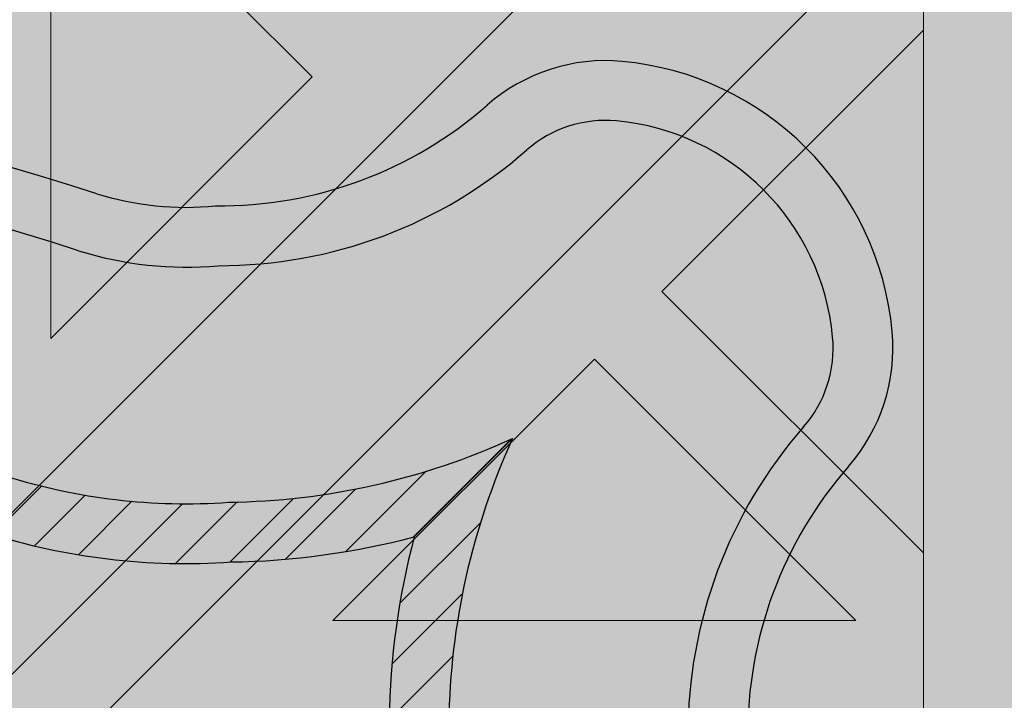
# Model space of a CAD drawing. Units: inches. Extents: x 844 to 2234, y 346 to 1084.
# Tile 20 of 93: x 1124.911 to 1127.536, y 703.246 to 705.06. Entities that reach past the tile are written whole.
import ezdxf

# ---------------------------------------------------------------- set-up
doc = ezdxf.new("R2010")
doc.units = ezdxf.units.IN
doc.header["$MEASUREMENT"] = 0
for name, color, linetype, lineweight in [('A-ANNO-DIMS', 2, 'Continuous', 18), ('furniture', 8, 'Continuous', 18), ('RA-AP-01$0$INT', 35, 'Continuous', 5)]:
    doc.layers.add(name, color=color, linetype=linetype, lineweight=lineweight)
doc.layers.add('RA-AP-01$0$FURN', color=3, linetype='Continuous')
doc.layers.add('RA-AP-01$0$WOOD', color=64, linetype='Continuous')
doc.styles.get("Standard").update_dxf_attribs({"font": 'arial.ttf'})
doc.dimstyles.get("Standard").update_dxf_attribs({"dimtxt": 6, "dimasz": 3, "dimexe": 0.18, "dimexo": 0.0625, "dimgap": 0.09, "dimtad": 0, "dimtih": 1, "dimtoh": 1, "dimdec": 1, "dimzin": 0, "dimdsep": 46, "dimlunit": 3, "dimtxsty": 'Standard', "dimblk": 'ARCHTICK', "dimcen": 0.09, "dimadec": 0, "dimazin": 0, "dimtfac": 1, "dimtdec": 1, "dimtofl": 0, "dimtmove": 0, "dimatfit": 3, "dimfxl": 1, "dimtolj": 1, "dimtzin": 0, "dimarcsym": 0})

# ---------------------------------------------------------------- blocks, each defined once
blk = doc.blocks.new('A$C18D01794')
at = {"layer": 'RA-AP-01$0$INT'}
blk.add_hatch(color=256, dxfattribs=at).paths.add_polyline_path([(4.505206456958071, -7.906712009588039), (5.305206456958072, -7.906712009588039), (5.305206456958072, -7.106712009588038), (5.255206456951893, -7.106712009588036), (5.25520645694868, -7.856712009570104), (4.555206456959269, -7.856712009588616), (4.555206456956052, -7.106712009588038), (4.505206456958073, -7.106712009588038)])
h = blk.add_hatch(color=256, dxfattribs=at)
h.paths.add_polyline_path([(4.585917135068448, -7.856712009587804), (4.614201406330596, -7.856712009587056), (4.668846067270487, -7.802067348644738), (4.723490728212344, -7.856712009584164), (4.771774999457151, -7.856712009582887), (4.826419660396886, -7.80206734864072), (4.862780050090322, -7.838427738332541), (4.844495778842715, -7.856712009580965), (4.862780050090411, -7.856712009580482), (4.905206456960182, -7.814285602707865), (4.947632863832445, -7.856712009578238), (4.965917135079675, -7.856712009577755), (4.947632863831759, -7.838427738330656), (4.983993253523576, -7.802067348637219), (5.038637914464627, -7.856712009575829), (5.08692218571208, -7.856712009574554), (5.141566846649976, -7.802067348634224), (5.196211507589851, -7.856712009571666), (5.224495778822615, -7.856712009570916), (4.905206456953975, -7.537422687702283)])
h.paths.add_polyline_path([(4.895206456956031, -7.575706958950402), (4.895206456958921, -7.684996280828174), (4.840561796018589, -7.630351619890275)], flags=16)
h.paths.add_polyline_path([(4.915206456955638, -7.575706958949956), (4.969851117895509, -7.630351619887399), (4.915206456957609, -7.684996280827732)], flags=16)
h.paths.add_polyline_path([(4.826419660395175, -7.644493755514321), (4.881064321335613, -7.699138416452331), (4.771774999456703, -7.69913841645522)], flags=16)
h.paths.add_polyline_path([(4.983993253519558, -7.644493755510815), (5.038637914460456, -7.699138416449285), (4.929348592581548, -7.69913841645126)], flags=16)
h.paths.add_polyline_path([(4.881064321336025, -7.719138416452334), (4.826419660397532, -7.773783077393256), (4.771774999457062, -7.719138416455217)], flags=16)
h.paths.add_polyline_path([(4.929348592582019, -7.71913841645126), (5.038637914460982, -7.719138416449284), (4.983993253522945, -7.773783077389749)], flags=16)
h.paths.add_polyline_path([(4.895206456960191, -7.733280552075633), (4.895206456962115, -7.806001331460164), (4.876922185715016, -7.824285602708492), (4.840561796021581, -7.787925213016675)], flags=16)
h.paths.add_polyline_path([(4.915206456958487, -7.733280552075187), (4.969851117899527, -7.787925213013798), (4.933490728206909, -7.824285602708034), (4.9152064569598, -7.806001331461736)], flags=16)
h.paths.add_polyline_path([(4.757632863832376, -7.733280552079264), (4.812277524772842, -7.787925213017304), (4.757632863834348, -7.842569873958233)], flags=16)
h.paths.add_polyline_path([(4.737632863832376, -7.73328055207979), (4.737632863834348, -7.842569873958701), (4.682988202893906, -7.787925213020692)], flags=16)
h.paths.add_polyline_path([(5.05278005008503, -7.733280552072701), (5.052780050087917, -7.842569873951664), (4.998135389146995, -7.787925213013169)], flags=16)
h.paths.add_polyline_path([(5.072780050085024, -7.733280552072333), (5.127424711025931, -7.787925213010806), (5.072780050087916, -7.842569873951244)], flags=16)
h.paths.add_polyline_path([(4.935917135072783, -7.506712009583784), (5.255206456948811, -7.826001331459767), (5.255206456948932, -7.797717060211899), (5.200561796010279, -7.743072399273238), (5.255206456949403, -7.688427738334128), (5.25520645694961, -7.640143467086677), (5.200561796009787, -7.585498806146837), (5.236922185702417, -7.549138416454212), (5.255206456949919, -7.56742268770172), (5.255206456949998, -7.549138416454178), (5.212780050078687, -7.506712009583814), (5.25520645695036, -7.464285602712145), (5.255206456950438, -7.446001331464763), (5.236922185702424, -7.464285602712779), (5.200561796009796, -7.427925213020149), (5.255206456950753, -7.373280552079203), (5.25520645695096, -7.324996280834394), (5.200561796010322, -7.270351619893748), (5.255206456951428, -7.215706958952649), (5.255206456951547, -7.187422687705071)])
h.paths.add_polyline_path([(5.042988202883395, -7.42792521302065), (5.097632863823085, -7.373280552080975), (5.097632863822622, -7.482569873959883)], flags=16)
h.paths.add_polyline_path([(5.028846067259663, -7.442067348644384), (5.083490728198774, -7.496712009583504), (4.974201406321001, -7.496712009583035)], flags=16)
h.paths.add_polyline_path([(5.117632863823087, -7.37328055208089), (5.172277524762331, -7.42792521302015), (5.11763286382262, -7.482569873959851)], flags=16)
h.paths.add_polyline_path([(5.08349072819877, -7.516712009582191), (5.028846067259652, -7.571356670521302), (4.974201406320998, -7.516712009582638)], flags=16)
h.paths.add_polyline_path([(5.131774999446817, -7.35913841645716), (5.186419660386065, -7.413783077396415), (5.241064321325782, -7.359138416456712)], flags=17)
h.paths.add_polyline_path([(5.131774999446228, -7.496712009583703), (5.186419660386065, -7.442067348643883), (5.222780050079488, -7.478427738337313), (5.204495778832781, -7.496712009584014)], flags=16)
h.paths.add_polyline_path([(5.097632863822613, -7.530854145205813), (5.097632863823061, -7.640143467084723), (5.042988202883383, -7.585498806145032)], flags=16)
h.paths.add_polyline_path([(5.131774999446899, -7.339138416457162), (5.241064321325809, -7.339138416456712), (5.186419660386591, -7.284493755517479)], flags=17)
h.paths.add_polyline_path([(5.131774999446226, -7.516712009581999), (5.204495778830767, -7.516712009581702), (5.22278005007868, -7.534996280829206), (5.186419660386049, -7.571356670521828)], flags=16)
h.paths.add_polyline_path([(5.11763286382262, -7.530854145205852), (5.17227752476232, -7.585498806145562), (5.117632863823064, -7.64014346708481)], flags=16)
h.paths.add_polyline_path([(5.186419660386069, -7.599640941770585), (5.241064321325754, -7.654285602710281), (5.131774999446791, -7.654285602709814)], flags=16)
h.paths.add_polyline_path([(5.131774999446872, -7.674285602709813), (5.24106432132578, -7.674285602710282), (5.186419660386554, -7.728930263649504)], flags=16)
h.paths.add_polyline_path([(5.255206456951811, -7.126001331467467), (5.255206456951895, -7.106712009588038), (4.555206456956052, -7.106712009588038), (4.555206456956136, -7.12600133146746), (4.905206456953973, -7.476001331465289)])
h.paths.add_polyline_path([(4.983993253513404, -7.368930263651977), (4.92934859257295, -7.314285602713969), (5.03863791445186, -7.314285602711063)], flags=16)
h.paths.add_polyline_path([(4.969851117889988, -7.383072399276016), (4.915206456952556, -7.437717060215906), (4.915206456949648, -7.328427738338133)], flags=16)
h.paths.add_polyline_path([(4.929348592572535, -7.294285602713971), (4.983993253511019, -7.239640941773039), (5.038637914451496, -7.294285602711065)], flags=16)
h.paths.add_polyline_path([(5.052780050074912, -7.280143467087016), (4.998135389134438, -7.225498806148989), (5.052780050072919, -7.170854145208052)], flags=16)
h.paths.add_polyline_path([(5.07278005007491, -7.280143467086489), (5.072780050072918, -7.170854145207579), (5.127424711013374, -7.225498806145578)], flags=16)
h.paths.add_polyline_path([(4.89520645695295, -7.437717060216355), (4.840561796013067, -7.383072399278919), (4.895206456950961, -7.328427738338582)], flags=16)
h.paths.add_polyline_path([(4.915206456948365, -7.280143467090674), (4.915206456946434, -7.207422687704125), (4.933490728192729, -7.18913841645701), (4.969851117886972, -7.225498806149623)], flags=16)
h.paths.add_polyline_path([(4.881064321327021, -7.314285602715054), (4.82641966038902, -7.368930263655506), (4.771774999448108, -7.314285602717047)], flags=16)
h.paths.add_polyline_path([(4.895206456950073, -7.280143467091125), (4.840561796009022, -7.225498806152518), (4.876922185700835, -7.18913841645908), (4.895206456948749, -7.207422687706589)], flags=16)
h.paths.add_polyline_path([(4.983993253510392, -7.211356670525576), (4.947632863816944, -7.174996280833758), (4.965917135064043, -7.156712009585847), (5.038637914448995, -7.156712009584522)], flags=16)
h.paths.add_polyline_path([(4.881064321326543, -7.294285602715056), (4.771774999447578, -7.294285602717046), (4.826419660385607, -7.239640941776569)], flags=16)
h.paths.add_polyline_path([(4.905206456946447, -7.19913841645844), (4.862780050074785, -7.156712009587725), (4.947632863816685, -7.156712009586302)], flags=16)
h.paths.add_polyline_path([(5.14156684663679, -7.211356670521528), (5.086922185696452, -7.156712009583639), (5.196211507574223, -7.156712009581651)], flags=16)
h.paths.add_polyline_path([(4.8264196603837, -7.211356670529104), (4.771774999442643, -7.156712009590501), (4.8444957788276, -7.156712009588568), (4.862780050075511, -7.17499628083566)], flags=16)
h.paths.add_polyline_path([(4.812277524760289, -7.225498806153156), (4.757632863822258, -7.28014346709363), (4.757632863819352, -7.170854145214669)], flags=16)
h.paths.add_polyline_path([(4.73763286382226, -7.280143467093997), (4.682988202881349, -7.22549880615554), (4.737632863819352, -7.170854145215086)], flags=16)
h.paths.add_polyline_path([(4.723490728195188, -7.156712009591787), (4.668846067257299, -7.211356670532127), (4.614201406317417, -7.156712009594693)], flags=16)
h.paths.add_polyline_path([(4.597632863829262, -7.506712009583814), (4.555206456957951, -7.54913841645418), (4.555206456958029, -7.56742268770172), (4.573490728205535, -7.549138416454212), (4.609851117898167, -7.585498806146839), (4.555206456958338, -7.640143467086675), (4.555206456958546, -7.688427738334125), (4.60985111789767, -7.743072399273238), (4.555206456959015, -7.797717060211899), (4.555206456959138, -7.826001331459767), (4.874495778835167, -7.506712009583786), (4.5552064569564, -7.187422687705062), (4.555206456956523, -7.215706958952644), (4.609851117897629, -7.270351619893746), (4.555206456956988, -7.324996280834396), (4.555206456957198, -7.373280552079195), (4.609851117898153, -7.427925213020147), (4.573490728205528, -7.464285602712779), (4.555206456957507, -7.446001331464756), (4.555206456957585, -7.464285602712143)])
h.paths.add_polyline_path([(4.712780050085332, -7.482569873959882), (4.712780050084863, -7.373280552080972), (4.767424711024555, -7.42792521302065)], flags=16)
h.paths.add_polyline_path([(4.726922185709173, -7.496712009583504), (4.781566846648288, -7.442067348644384), (4.836211507586949, -7.496712009583033)], flags=16)
h.paths.add_polyline_path([(4.692780050085327, -7.482569873959851), (4.638135389145619, -7.427925213020149), (4.692780050084865, -7.373280552080892)], flags=16)
h.paths.add_polyline_path([(4.726922185709182, -7.516712009582191), (4.836211507586949, -7.51671200958264), (4.7815668466483, -7.571356670521304)], flags=16)
h.paths.add_polyline_path([(4.678637914461726, -7.496712009583706), (4.605917135075169, -7.496712009584014), (4.587632863828464, -7.478427738337311), (4.623993253521887, -7.442067348643881)], flags=16)
h.paths.add_polyline_path([(4.712780050085336, -7.530854145205816), (4.767424711024568, -7.585498806145034), (4.71278005008489, -7.640143467084724)], flags=16)
h.paths.add_polyline_path([(4.678637914461726, -7.516712009582001), (4.623993253521899, -7.571356670521829), (4.587632863829271, -7.534996280829206), (4.605917135077185, -7.5167120095817)], flags=16)
h.paths.add_polyline_path([(4.692780050085336, -7.530854145205848), (4.692780050084889, -7.64014346708481), (4.638135389145632, -7.585498806145562)], flags=16)
h.paths.add_polyline_path([(4.623993253521885, -7.413783077396415), (4.678637914461131, -7.359138416457161), (4.56934859258217, -7.359138416456712)], flags=17)
h.paths.add_polyline_path([(4.623993253521901, -7.599640941770568), (4.678637914461158, -7.654285602709814), (4.569348592582195, -7.654285602710281)], flags=16)
h.paths.add_polyline_path([(4.678637914461051, -7.339138416457162), (4.623993253521361, -7.284493755517479), (4.569348592582143, -7.339138416456712)], flags=17)
h.paths.add_polyline_path([(4.678637914461076, -7.674285602709813), (4.623993253521399, -7.728930263649504), (4.569348592582167, -7.674285602710281)], flags=16)
h = blk.add_hatch(color=256, dxfattribs=at)
h.paths.add_polyline_path([(4.905206456954232, -7.537422687702028), (4.874495778835232, -7.506712009583718), (4.555206456959138, -7.826001331459766), (4.555206456959269, -7.856712009588616), (4.585917135068449, -7.856712009587804)])
h.paths.add_polyline_path([(4.935917135072152, -7.506712009583152), (4.905206456953497, -7.537422687701806), (5.224495778822614, -7.856712009570917), (5.255206456948681, -7.856712009570104), (5.255206456948813, -7.826001331459768)])
h.paths.add_polyline_path([(5.255206456951549, -7.18742268770507), (5.255206456951813, -7.126001331467461), (4.905206456953563, -7.476001331465701), (4.935917135072559, -7.506712009584006)])
h.paths.add_polyline_path([(4.874495778835167, -7.506712009583785), (4.905206456953818, -7.476001331465132), (4.555206456956135, -7.126001331467458), (4.555206456956399, -7.187422687705064)])
h = blk.add_hatch(color=256, dxfattribs=at)
h.paths.add_polyline_path([(5.028846067259997, -7.571356670520955), (4.974201406321342, -7.516712009582294), (5.083490728199115, -7.516712009581846)])
h.paths.add_polyline_path([(4.974201406321344, -7.496712009582688), (5.028846067260004, -7.442067348644037), (5.083490728199117, -7.496712009583157)])
h.paths.add_polyline_path([(5.042988202883738, -7.427925213020309), (5.097632863823428, -7.373280552080627), (5.097632863822963, -7.482569873959537)])
h.paths.add_polyline_path([(5.117632863822961, -7.482569873959509), (5.117632863823428, -7.373280552080546), (5.172277524762674, -7.427925213019804)])
h.paths.add_polyline_path([(5.131774999446572, -7.496712009583358), (5.186419660386406, -7.442067348643536), (5.222780050079831, -7.478427738336961), (5.204495778833122, -7.496712009583667)])
h.paths.add_polyline_path([(5.236922185702764, -7.464285602712433), (5.200561796010139, -7.427925213019802), (5.255206456949971, -7.373280552079975), (5.255206456950271, -7.446001331464927)])
h.paths.add_polyline_path([(5.186419660386412, -7.41378307739607), (5.131774999447164, -7.359138416456815), (5.241064321326123, -7.359138416456366)])
h.paths.add_polyline_path([(5.131774999447238, -7.339138416456815), (5.186419660386934, -7.284493755517132), (5.241064321326153, -7.339138416456368)])
h.paths.add_polyline_path([(5.200561796010663, -7.270351619893402), (5.255206456949324, -7.215706958954747), (5.255206456949777, -7.324996280832518)])
h.paths.add_polyline_path([(5.21278005007903, -7.50671200958347), (5.255206456950223, -7.464285602712278), (5.255206456950696, -7.549138416454185)])
h.paths.add_polyline_path([(5.13177499944657, -7.516712009581652), (5.204495778831106, -7.516712009581354), (5.222780050079024, -7.534996280828858), (5.186419660386397, -7.571356670521485)])
h.paths.add_polyline_path([(5.117632863823405, -7.640143467084465), (5.117632863822955, -7.530854145205498), (5.172277524762665, -7.585498806145217)])
h.paths.add_polyline_path([(5.042988202883727, -7.585498806144689), (5.097632863822957, -7.530854145205474), (5.097632863823407, -7.64014346708438)])
h.paths.add_polyline_path([(5.131774999447135, -7.654285602709467), (5.186419660386394, -7.599640941770219), (5.241064321326097, -7.654285602709933)])
h.paths.add_polyline_path([(5.200561796010128, -7.585498806146492), (5.236922185702758, -7.549138416453866), (5.255206456950264, -7.567422687701371), (5.255206456949948, -7.640143467086325)])
h.paths.add_polyline_path([(5.186419660386895, -7.728930263649157), (5.131774999447213, -7.674285602709467), (5.241064321326127, -7.674285602709934)])
h.paths.add_polyline_path([(5.200561796010624, -7.743072399272893), (5.255206456949745, -7.688427738333778), (5.255206456949276, -7.797717060211553)])
h = blk.add_hatch(color=256, dxfattribs=at)
h.paths.add_polyline_path([(4.969851117891331, -7.630351619889621), (4.915206456952669, -7.575706958950966), (4.915206456952222, -7.684996280828739)])
h.paths.add_polyline_path([(4.895206456953064, -7.575706958950968), (4.840561796014413, -7.630351619889628), (4.895206456953533, -7.684996280828741)])
h.paths.add_polyline_path([(4.826419660390684, -7.644493755513362), (4.771774999451003, -7.699138416453052), (4.881064321329913, -7.699138416452587)])
h.paths.add_polyline_path([(4.881064321329884, -7.719138416452585), (4.771774999450921, -7.719138416453052), (4.82641966039018, -7.773783077392298)])
h.paths.add_polyline_path([(4.895206456953734, -7.733280552076196), (4.840561796013912, -7.787925213016031), (4.876922185707337, -7.824285602709455), (4.895206456954043, -7.806001331462747)])
h.paths.add_polyline_path([(4.862780050082808, -7.838427738332388), (4.826419660390178, -7.802067348639763), (4.771774999450351, -7.856712009579595), (4.844495778835303, -7.856712009579895)])
h.paths.add_polyline_path([(4.812277524766446, -7.787925213016036), (4.757632863827191, -7.733280552076788), (4.757632863826741, -7.842569873955747)])
h.paths.add_polyline_path([(4.737632863827191, -7.733280552076863), (4.682988202887508, -7.787925213016558), (4.737632863826743, -7.842569873955778)])
h.paths.add_polyline_path([(4.668846067263777, -7.802067348640287), (4.614201406325123, -7.856712009578949), (4.723490728202894, -7.856712009579402)])
h.paths.add_polyline_path([(4.905206456953846, -7.814285602708654), (4.862780050082654, -7.856712009579847), (4.947632863824561, -7.85671200958032)])
h.paths.add_polyline_path([(4.915206456952028, -7.733280552076195), (4.91520645695173, -7.806001331460731), (4.933490728199234, -7.824285602708648), (4.96985111789186, -7.787925213016022)])
h.paths.add_polyline_path([(5.038637914454841, -7.719138416453029), (4.929348592575874, -7.71913841645258), (4.983993253515593, -7.773783077392289)])
h.paths.add_polyline_path([(4.983993253515065, -7.644493755513352), (4.929348592575849, -7.699138416452582), (5.038637914454755, -7.699138416453031)])
h.paths.add_polyline_path([(5.052780050079843, -7.73328055207676), (4.998135389140595, -7.787925213016018), (5.052780050080309, -7.842569873955721)])
h.paths.add_polyline_path([(4.983993253516868, -7.802067348639752), (4.947632863824241, -7.838427738332383), (4.965917135071747, -7.856712009579888), (5.038637914456701, -7.856712009579572)])
h.paths.add_polyline_path([(5.127424711019533, -7.787925213016519), (5.072780050079843, -7.733280552076838), (5.07278005008031, -7.842569873955751)])
h.paths.add_polyline_path([(5.141566846643269, -7.802067348640248), (5.086922185704154, -7.85671200957937), (5.196211507581929, -7.856712009578901)])
for p, q in [((5.255206456951895, -7.106712009588038), (5.255206456948681, -7.856712009570104)), ((4.935917135072783, -7.506712009583784), (5.255206456948813, -7.826001331459769)), ((4.905206456953975, -7.537422687702283), (5.224495778822613, -7.856712009570916)), ((5.131774999446872, -7.674285602709813), (5.241064321325782, -7.674285602710281)), ((5.18641966038655, -7.728930263649502), (5.131774999446872, -7.674285602709813)), ((5.241064321325782, -7.674285602710281), (5.186419660386552, -7.728930263649504)), ((5.255206456949399, -7.68842773833413), (5.200561796010281, -7.743072399273238)), ((5.12742471102593, -7.787925213010804), (5.072780050085028, -7.733280552072336)), ((5.072780050085028, -7.733280552072336), (5.072780050087916, -7.842569873951246)), ((5.255206456948934, -7.797717060211899), (5.200561796010281, -7.743072399273238)), ((5.072780050087916, -7.842569873951246), (5.127424711025931, -7.787925213010806))]:
    blk.add_line(p, q, dxfattribs=at)
blk = doc.blocks.new('A$C32926AE1')
at = {"layer": 'RA-AP-01$0$WOOD'}
h = blk.add_hatch(color=256, dxfattribs=at)
h.dxf.hatch_style = 1
h.paths.add_polyline_path([(5.157430609644524, 4.573483066760929, -0.1009492694046607), (5.155401577623758, 4.593365984175333, -0.1842662638101597), (5.172249623284174, 4.638795604568598, 0.2056608120311276), (5.179560981299304, 4.661316324430096, 0.3614336704623542), (5.134352340494423, 4.706524965234944, 0.2056608120311297), (5.111831620632933, 4.699213607219793, -0.1842662638101113), (5.066402000239693, 4.682365561559342, -0.1055311479399994), (5.045656153913092, 4.68467289944697, 0.1567636581983829), (4.763886414745334, 4.684672899446966, -0.1055311479399895), (4.743140568418733, 4.68236556155934, -0.1842662638100833), (4.6977109480255, 4.69921360721979, 0.2056608120302612), (4.675190228164109, 4.706524965234949, 0.3614336704708441), (4.629981587358889, 4.66131632442871, 0.2056608120245944), (4.637292945374126, 4.638795604567974, -0.1842662638101024), (4.654140991034615, 4.59336598417475, -0.1009492694055169), (4.652111959013835, 4.573483066760181, 0.021410119221476), (4.629748025606143, 4.156712009541676, 0.0214101192214795), (4.652111959013809, 3.739940952323101, -0.1009492694059586), (4.654140991034615, 3.720058034908448, -0.1842662638100975), (4.637292945374126, 3.674628414515226, 0.2056608120245705), (4.629981587358889, 3.652107694654492, 0.3614336704708879), (4.675190228164113, 3.606899053848249, 0.2056608120302384), (4.697710948025501, 3.614210411863408, -0.1842662638100995), (4.743140568418738, 3.63105845752386, -0.1055311479402541), (4.763886414745388, 3.628751119636215, 0.1567636581983776), (5.045656153913137, 3.628751119636244, -0.1055311479397538), (5.066402000239692, 3.631058457523857, -0.1842662638101067), (5.111831620632931, 3.614210411863407, 0.2056608120310924), (5.134352340494417, 3.606899053848256, 0.3614336704624001), (5.179560981299307, 3.652107694653103, 0.2056608120311314), (5.172249623284175, 3.6746284145146, -0.1842662638101402), (5.155401577623758, 3.72005803490786, -0.1009492694051366), (5.15743060964455, 3.739940952322354, 0.0214101192215073), (5.179794543052287, 4.156712009541468, 0.0214101192215252)])
h.paths.add_polyline_path([(4.639748609479751, 4.156712009541513, 0.0213537860821624), (4.661970494867118, 3.741887061152232, -0.094075836301374), (4.664143710413708, 3.7196126951003, -0.1824818158568985), (4.644813765429836, 3.668037719127816, 0.2056608120245319), (4.639939526753007, 3.653023905887301, 0.3614336704710246), (4.676106439397173, 3.616856993242342, 0.2056608120302234), (4.691120252638095, 3.621731231919122, -0.1824818158602558), (4.742695228611606, 3.641061176902986, -0.1029891339458722), (4.766991894714349, 3.638256818950944, 0.156709409989566), (5.042550673941472, 3.638256818950105, -0.102989133958497), (5.066847340047078, 3.641061176902949, -0.1824818158594995), (5.118422316020358, 3.621731231919103, 0.2056608120311416), (5.133436129261316, 3.616856993242346, 0.3614336704621468), (5.169603041905217, 3.653023905886178, 0.2056608120310986), (5.164728803228477, 3.668037719127177, -0.1824818158565612), (5.145398858244737, 3.719612695099578, -0.0940758363009313), (5.147572073791232, 3.741887061151398, 0.0213537860822023), (5.169793959178681, 4.156712009541451, 0.0213537860822226), (5.147572073791203, 4.571536957931898, -0.0940758363005034), (5.145398858244737, 4.59381132398362, -0.1824818158565587), (5.164728803228476, 4.645386299956021, 0.2056608120311045), (5.169603041905216, 4.66040011319702, 0.3614336704621845), (5.133436129261313, 4.696567025840856, 0.2056608120310773), (5.118422316020359, 4.691692787164098, -0.182481815859508), (5.066847340047078, 4.67236284218025, -0.1029891339584606), (5.04255067394148, 4.675167200133092, 0.156709409989566), (4.766991894714357, 4.675167200132257, -0.1029891339458842), (4.742695228611611, 4.672362842180213, -0.1824818158602725), (4.691120252638095, 4.691692787164077, 0.2056608120302152), (4.676106439397174, 4.696567025840858, 0.3614336704710363), (4.639939526753005, 4.660400113195899, 0.2056608120245495), (4.644813765429837, 4.645386299955384, -0.1824818158568934), (4.664143710413708, 4.593811323982902, -0.0940758363009187), (4.661970494867149, 4.571536957931074, 0.021353786082177)], flags=16)
h.paths.add_polyline_path([(5.129794543052235, 4.432167055276933, -0.0141661062790638), (5.130152669293814, 4.156927903047693, -0.0141661062790647), (5.129794543052234, 3.881688750818433, -0.0785247771143638), (5.10979738006795, 3.755143611847103, 0.0945969212073497), (5.105408519571111, 3.717898134952927, 0.1043170707844957), (5.116074640131521, 3.670385395016088, 0.1043170707864965), (5.068561900193738, 3.681051515576561, 0.09459692119553), (5.031316423304057, 3.676662655080835, -0.1580239521427272), (4.778226145355827, 3.676662655080367, 0.0945969211986668), (4.740980668464973, 3.681051515576592, 0.1043170707882822), (4.693467928526415, 3.670385395015844, 0.1043170707867916), (4.704134049087309, 3.717898134953662, 0.0945969211972894), (4.69974518859162, 3.755143611844042, -0.0785247771163196), (4.679748025606343, 3.881688750818406, -0.0141661062790663), (4.679389899364763, 4.156927903047693, -0.0141661062790672), (4.679748025606343, 4.432167055276998, -0.0785247771163064), (4.699745188591625, 4.55871219425134, 0.094596921197333), (4.704134049087308, 4.595957671141738, 0.1043170707867205), (4.693467928526416, 4.643470411079523, 0.1043170707882628), (4.740980668464965, 4.632804290518776, 0.0945969211988114), (4.778226145355874, 4.637193151015016, -0.158023952142669), (5.031316423304015, 4.637193151014546, 0.0945969211956361), (5.068561900193736, 4.632804290518806, 0.1043170707864979), (5.11607464013152, 4.643470411079278, 0.1043170707844617), (5.105408519571112, 4.595957671142455, 0.0945969212074597), (5.109797380067959, 4.558712194248236, -0.0785247771143467)], flags=0)
h.paths.add_polyline_path([(5.119794532311105, 4.432259799204851, -0.0142000800617244), (5.120156169157484, 4.156927903047701, -0.0142000800617277), (5.119794532311105, 3.881596006890482, -0.0784894509520253), (5.100273383573699, 3.758192358677797, 0.0940138827242913), (5.095413455884425, 3.717477693979438, 0.0606271852308753), (5.099615656341024, 3.686844378806616, 0.0606271852322524), (5.068982341167493, 3.691046579263239, 0.0940138827010453), (5.028267676478798, 3.686186651576848, -0.1580706864508061), (4.781274892180912, 3.686186651576435, 0.0940138827026903), (4.740560227491556, 3.691046579263279, 0.0606271852339895), (4.709926912317155, 3.686844378806508, 0.0606271852329405), (4.714129112773991, 3.717477693980356, 0.094013882701304), (4.709269185087677, 3.758192358669163, -0.0784894509577193), (4.689748036347473, 3.881596006890469, -0.014200080061729), (4.689386399501094, 4.156927903047709, -0.0142000800617217), (4.689748036347473, 4.432259799204808, -0.078489450957724), (4.709269185087651, 4.555663447426125, 0.0940138827014585), (4.714129112773992, 4.596378112114996, 0.0606271852329731), (4.709926912317154, 4.62701142728886, 0.0606271852340196), (4.74056022749157, 4.622809226832087, 0.0940138827024997), (4.781274892180847, 4.627669154518912, -0.1580706864508359), (5.028267676478777, 4.627669154518526, 0.0940138827010946), (5.068982341167492, 4.622809226832129, 0.060627185232254), (5.099615656341024, 4.627011427288751, 0.0606271852308727), (5.095413455884425, 4.59637811211593, 0.0940138827241088), (5.100273383573675, 4.555663447417647, -0.0784894509520978)], flags=0)
h.paths.add_polyline_path([(5.06978912287499, 4.430218106756144, -0.014241683694547), (5.070173729147532, 4.156927903047672, -0.0142416836945458), (5.06978912287499, 3.883637699339223, -0.0800609523125196), (5.052662118612511, 3.773463122773442, 0.0526421978001116), (5.04590916754064, 3.740550867606997, 0.0526421977992423), (5.012996912374707, 3.73379791653534, -0.1583028414718258), (4.796545656286308, 3.73379791653451, 0.0526421978034211), (4.763633401117837, 3.740550867607021, 0.0526421978018622), (4.756880450045755, 3.773463122774558, -0.0800609523117106), (4.739753445783639, 3.883637699339268, -0.0142416836945435), (4.739368839511098, 4.156927903047671, -0.0142416836945477), (4.739753445783639, 4.430218106756155, -0.0800609523116345), (4.75688045004574, 4.540392683320762, 0.052642197801941), (4.763633401117837, 4.573304938488346, 0.0526421978035071), (4.796545656286361, 4.580057889560873, -0.1583028414717561), (5.012996912374669, 4.580057889560039, 0.0526421977993048), (5.04590916754064, 4.57330493848837, 0.0526421978002057), (5.052662118612529, 4.540392683321868, -0.080060952312477)], flags=0)
h.paths.add_polyline_path([(5.049789715110557, 4.43038092723357, -0.0143097550741839), (5.05018085590259, 4.156927903047715, -0.0143097550741854), (5.049789715110558, 3.883474878861827, -0.0800685599149176), (5.03362098255317, 3.779581877367999, 0.0306258898956367), (5.028241146483733, 3.758218888663947, 0.0306258898977031), (5.006878157778253, 3.75283905259408, -0.1583983521624096), (4.802664410878162, 3.752839052594731, 0.0306258898946014), (4.781301422174808, 3.758218888663924, 0.0306258898967912), (4.775921586105202, 3.779581877368794, -0.080068559914251), (4.759752853548071, 3.883474878861786, -0.0143097550741854), (4.759361712756037, 4.156927903047671, -0.0143097550741854), (4.759752853548071, 4.430380927233557, -0.0800685599142479), (4.775921586105193, 4.534273928726546, 0.0306258898968306), (4.781301422174808, 4.555636917431444, 0.0306258898945754), (4.802664410878143, 4.561016753500631, -0.1583983521624168), (5.006878157778244, 4.561016753501291, 0.0306258898977177), (5.028241146483733, 4.555636917431421, 0.0306258898958182), (5.03362098255321, 4.534273928727244, -0.080068559914796)], flags=0)
h.paths.add_polyline_path([(4.999766070382627, 4.428171244713864, -0.0143443147609634), (5.000198441819402, 4.156927903047689, -0.0143443147609612), (4.999766070382627, 3.885684561381556, -0.0784641635803329), (4.987356730658798, 3.799103304488872, -0.1506053783831347), (4.822185837999821, 3.79910330448882, -0.0784641635803318), (4.809776498276007, 3.885684561381509, -0.014344314760963), (4.809344126839227, 4.156927903047677, -0.0143443147609645), (4.809776498276007, 4.428171244713873, -0.0784641635803192), (4.822185837999822, 4.514752501606549, -0.1506053783831338), (4.987356730658798, 4.514752501606494, -0.078464163580285)], flags=0)
h.paths.add_polyline_path([(4.979755254238824, 4.42764379880488, -0.0143772539198268), (4.980205517789977, 4.156927903047693, -0.0143772539198275), (4.979755254238824, 3.886212007290489, -0.0689242507424422), (4.971183264704897, 3.815276770442801, -0.1296645318904179), (4.838359303953726, 3.815276770442746, -0.0689242507424186), (4.829787314419809, 3.886212007290419, -0.0143772539198292), (4.829337050868653, 4.156927903047653, -0.0143772539198325), (4.829787314419809, 4.427643798804946, -0.0689242507424211), (4.838359303953725, 4.498579035652621, -0.1296645318904187), (4.971183264704897, 4.498579035652565, -0.0689242507424401)], flags=0)
h = blk.add_hatch(color=256, dxfattribs=at)
h.dxf.hatch_style = 1
h.paths.add_polyline_path([(5.145398858244737, 4.59381132398362, -0.1824818158565616), (5.164728803228476, 4.645386299956021, 0.2056608120311045), (5.169603041905216, 4.66040011319702, 0.3614336704621845), (5.133436129261313, 4.696567025840856, 0.2056608120310773), (5.118422316020359, 4.691692787164098, -0.182481815859508), (5.066847340047078, 4.67236284218025, -0.1029891339584606), (5.04255067394148, 4.675167200133092, 0.156709409989566), (4.766991894714357, 4.675167200132257, -0.1029891339458842), (4.742695228611611, 4.672362842180213, -0.1824818158602725), (4.691120252638095, 4.691692787164077, 0.2056608120302152), (4.676106439397174, 4.696567025840858, 0.3614336704710363), (4.639939526753005, 4.660400113195899, 0.2056608120245495), (4.644813765429837, 4.645386299955384, -0.1824818158568934), (4.664143710413708, 4.593811323982902, -0.0940758363009187), (4.661970494867149, 4.571536957931074, 0.0213537860821772), (4.639748609479751, 4.156712009541507, 0.0213537860821625), (4.661970494867119, 3.741887061152226, -0.0940758363013071), (4.664143710413708, 3.719612695100309, -0.1824818158569294), (4.644813765429836, 3.668037719127816, 0.2056608120245319), (4.639939526753007, 3.653023905887301, 0.3614336704710246), (4.676106439397173, 3.616856993242342, 0.2056608120302234), (4.691120252638095, 3.621731231919122, -0.1824818158602558), (4.742695228611606, 3.641061176902986, -0.1029891339458722), (4.766991894714349, 3.638256818950944, 0.156709409989566), (5.042550673941472, 3.638256818950105, -0.102989133958497), (5.066847340047078, 3.641061176902949, -0.1824818158594995), (5.118422316020358, 3.621731231919103, 0.2056608120311416), (5.133436129261316, 3.616856993242346, 0.3614336704621468), (5.169603041905217, 3.653023905886178, 0.2056608120310986), (5.164728803228477, 3.668037719127177, -0.1824818158565612), (5.145398858244737, 3.719612695099578, -0.0940758363009313), (5.147572073791232, 3.741887061151398, 0.0213537860822023), (5.169793959178681, 4.156712009541451, 0.0213537860822226), (5.147572073791203, 4.571536957931898, -0.0940758363004996)])
h.paths.add_polyline_path([(5.109797380067958, 4.55871219424824, -0.0785247771143472), (5.129794543052234, 4.432167055276936, -0.0141661062790644), (5.130152669293814, 4.156927903047685, -0.014166106279066), (5.129794543052234, 3.881688750818401, -0.0785247771143517), (5.109797380067946, 3.755143611847092, 0.0945969212073132), (5.105408519571111, 3.717898134952929, 0.1043170707844995), (5.116074640131521, 3.670385395016088, 0.1043170707864965), (5.068561900193738, 3.681051515576561, 0.09459692119553), (5.031316423304057, 3.676662655080835, -0.1580239521427272), (4.778226145355827, 3.676662655080367, 0.0945969211986668), (4.740980668464973, 3.681051515576592, 0.1043170707882822), (4.693467928526415, 3.670385395015844, 0.1043170707867916), (4.704134049087309, 3.717898134953662, 0.0945969211972894), (4.69974518859162, 3.755143611844042, -0.0785247771163196), (4.679748025606343, 3.881688750818406, -0.0141661062790663), (4.679389899364763, 4.156927903047693, -0.0141661062790672), (4.679748025606343, 4.432167055276998, -0.0785247771163064), (4.699745188591625, 4.55871219425134, 0.094596921197333), (4.704134049087308, 4.595957671141738, 0.1043170707867205), (4.693467928526416, 4.643470411079523, 0.1043170707882628), (4.740980668464965, 4.632804290518776, 0.0945969211988114), (4.778226145355874, 4.637193151015016, -0.158023952142669), (5.031316423304015, 4.637193151014546, 0.0945969211956361), (5.068561900193736, 4.632804290518806, 0.1043170707864979), (5.11607464013152, 4.643470411079278, 0.1043170707844617), (5.105408519571112, 4.595957671142455, 0.0945969212074504)], flags=16)
h.paths.add_polyline_path([(5.100273383573655, 4.55566344741771, -0.0784894509521388), (5.119794532311105, 4.432259799204852, -0.0142000800617252), (5.120156169157484, 4.156927903047686, -0.014200080061726), (5.119794532311105, 3.881596006890502, -0.0784894509520446), (5.100273383573696, 3.758192358677786, 0.0940138827242721), (5.095413455884425, 3.717477693979436, 0.0606271852308692), (5.099615656341024, 3.686844378806616, 0.0606271852322522), (5.068982341167493, 3.691046579263239, 0.0940138827010453), (5.028267676478798, 3.686186651576848, -0.1580706864508061), (4.781274892180912, 3.686186651576435, 0.0940138827026903), (4.740560227491556, 3.691046579263279, 0.0606271852339895), (4.709926912317155, 3.686844378806508, 0.0606271852329405), (4.714129112773991, 3.717477693980356, 0.094013882701304), (4.709269185087677, 3.758192358669163, -0.0784894509577193), (4.689748036347473, 3.881596006890469, -0.014200080061729), (4.689386399501094, 4.156927903047709, -0.0142000800617217), (4.689748036347473, 4.432259799204808, -0.078489450957724), (4.709269185087651, 4.555663447426125, 0.0940138827014585), (4.714129112773992, 4.596378112114996, 0.0606271852329731), (4.709926912317154, 4.62701142728886, 0.0606271852340196), (4.74056022749157, 4.622809226832087, 0.0940138827024997), (4.781274892180847, 4.627669154518912, -0.1580706864508359), (5.028267676478777, 4.627669154518526, 0.0940138827010946), (5.068982341167492, 4.622809226832129, 0.060627185232254), (5.099615656341024, 4.627011427288751, 0.0606271852308727), (5.095413455884425, 4.59637811211593, 0.094013882723957)], flags=0)
h.paths.add_polyline_path([(5.04590916754064, 4.57330493848837, 0.0526421978002057), (5.052662118612529, 4.540392683321868, -0.0800609523124783), (5.06978912287499, 4.430218106756142, -0.0142416836945469), (5.070173729147532, 4.156927903047672, -0.0142416836945458), (5.06978912287499, 3.883637699339223, -0.0800609523125196), (5.052662118612511, 3.773463122773442, 0.0526421978001116), (5.04590916754064, 3.740550867606997, 0.0526421977992423), (5.012996912374707, 3.73379791653534, -0.1583028414718258), (4.796545656286308, 3.73379791653451, 0.0526421978034211), (4.763633401117837, 3.740550867607021, 0.0526421978018622), (4.756880450045755, 3.773463122774558, -0.0800609523117106), (4.739753445783639, 3.883637699339268, -0.0142416836945435), (4.739368839511098, 4.156927903047671, -0.0142416836945477), (4.739753445783639, 4.430218106756155, -0.0800609523116345), (4.75688045004574, 4.540392683320762, 0.052642197801941), (4.763633401117837, 4.573304938488346, 0.0526421978035071), (4.796545656286361, 4.580057889560873, -0.1583028414717561), (5.012996912374669, 4.580057889560039, 0.0526421977993048)], flags=0)
h.paths.add_polyline_path([(5.028241146483733, 4.555636917431422, 0.0306258898956949), (5.033620982553182, 4.534273928727329, -0.0800685599148649), (5.049789715110557, 4.430380927233569, -0.0143097550741839), (5.05018085590259, 4.156927903047715, -0.0143097550741854), (5.049789715110558, 3.883474878861827, -0.0800685599149176), (5.03362098255317, 3.779581877367999, 0.0306258898956367), (5.028241146483733, 3.758218888663947, 0.0306258898977031), (5.006878157778253, 3.75283905259408, -0.1583983521624096), (4.802664410878162, 3.752839052594731, 0.0306258898946014), (4.781301422174808, 3.758218888663924, 0.0306258898967912), (4.775921586105202, 3.779581877368794, -0.080068559914251), (4.759752853548071, 3.883474878861786, -0.0143097550741854), (4.759361712756037, 4.156927903047671, -0.0143097550741854), (4.759752853548071, 4.430380927233557, -0.0800685599142479), (4.775921586105193, 4.534273928726546, 0.0306258898968306), (4.781301422174808, 4.555636917431444, 0.0306258898945754), (4.802664410878143, 4.561016753500631, -0.1583983521624168), (5.006878157778244, 4.561016753501291, 0.0306258898977174)], flags=0)
h.paths.add_polyline_path([(4.987356730658798, 4.514752501606494, -0.0784641635803018), (4.999766070382627, 4.428171244713845, -0.0143443147609637), (5.000198441819402, 4.156927903047665, -0.0143443147609622), (4.999766070382628, 3.885684561381514, -0.0784641635802952), (4.987356730658797, 3.799103304488872, -0.1506053783831338), (4.822185837999821, 3.799103304488819, -0.0784641635803342), (4.809776498276007, 3.885684561381512, -0.0143443147609628), (4.809344126839227, 4.156927903047676, -0.0143443147609646), (4.809776498276007, 4.428171244713873, -0.0784641635803192), (4.822185837999822, 4.514752501606549, -0.1506053783831338)], flags=0)
h.paths.add_polyline_path([(4.971183264704897, 4.498579035652566, -0.0689242507424384), (4.979755254238824, 4.427643798804883, -0.0143772539198276), (4.980205517789977, 4.15692790304768, -0.0143772539198258), (4.979755254238823, 3.88621200729051, -0.0689242507424628), (4.971183264704897, 3.815276770442801, -0.129664531890417), (4.838359303953726, 3.815276770442746, -0.0689242507424186), (4.829787314419809, 3.886212007290419, -0.0143772539198292), (4.829337050868653, 4.156927903047653, -0.0143772539198325), (4.829787314419809, 4.427643798804946, -0.0689242507424211), (4.838359303953725, 4.498579035652621, -0.1296645318904187)], flags=0)
h = blk.add_hatch(dxfattribs=at)
h.set_pattern_fill('ANSI31', color=256, scale=0.05, style=0)
h.set_pattern_definition([(45, (0, 0), (-0.0044194173824159, 0.0044194173824159), [])])
h.paths.add_polyline_path([(5.130152669293814, 4.156927903047704, 0.0141661062790657), (5.129794543052234, 4.432167055276982, 0.0777827904001433), (5.110168979996553, 4.557559993161921, -0.0976515123401879), (5.105408519571111, 4.595957671142454, -0.1043170707844687), (5.116074640131522, 4.64347041107928), (5.099615656341024, 4.627011427288751, 0.0606271852308727), (5.095413455884425, 4.59637811211593, 0.0940138827241088), (5.100273383573675, 4.555663447417647, -0.0784894509520972), (5.119794532311105, 4.432259799204852, -0.0142000800617252), (5.120156169157484, 4.156927903047686, -0.014200080061726), (5.119794532311105, 3.881596006890502, -0.0784894509520446), (5.100273383573696, 3.758192358677786, 0.0940138827242721), (5.095413455884425, 3.717477693979436, 0.0606271852308692), (5.099615656341024, 3.686844378806616), (5.116074640131519, 3.67038539501609, -0.1043170707844594), (5.105408519571112, 3.717898134952912, -0.0976515123401594), (5.11016897999655, 3.756295812933435, 0.0777827904001654), (5.129794543052234, 3.881688750818409, 0.0141661062790665)])
h.paths.add_polyline_path([(5.030164222210597, 3.676291055149937, -0.0976515123472002), (5.068561900193739, 3.681051515576561, -0.1043170707864927), (5.116074640131521, 3.670385395016088), (5.099615656341024, 3.686844378806616, 0.0606271852322522), (5.068982341167493, 3.691046579263239, 0.0940138827010453), (5.028267676478798, 3.686186651576848, -0.1580706864508061), (4.781274892180912, 3.686186651576435, 0.0940138827026903), (4.740560227491556, 3.691046579263279, 0.0606271852339913), (4.709926912317154, 3.686844378806508), (4.693467928526416, 3.670385395015845, -0.1043170707882796), (4.740980668464973, 3.681051515576592, -0.0976515123427246), (4.779378346446416, 3.676291055150394, 0.156512506893803)])
h.paths.add_polyline_path([(4.689748036347473, 3.881596006890472, -0.014200080061729), (4.689386399501094, 4.156927903047712, -0.0142000800617195), (4.689748036347473, 4.432259799204768, -0.078489450957742), (4.709269185087648, 4.555663447426114, 0.0940138827014821), (4.714129112773992, 4.596378112114995, 0.0606271852329748), (4.709926912317154, 4.62701142728886), (4.693467928526414, 4.643470411079524, -0.1043170707867939), (4.704134049087309, 4.595957671141706, -0.09765151234893), (4.699373588660725, 4.557559993157876, 0.0777827903975372), (4.679748025606343, 4.432167055276987, 0.0141661062790675), (4.679389899364763, 4.156927903047675, 0.0141661062790641), (4.679748025606343, 3.88168875081843, 0.0777827903975637), (4.699373588660724, 3.756295812937497, -0.0976515123490278), (4.704134049087308, 3.717898134953629, -0.1043170707867196), (4.693467928526416, 3.670385395015845), (4.709926912317155, 3.686844378806508, 0.0606271852329413), (4.714129112773991, 3.717477693980357, 0.0940138827013084), (4.709269185087676, 3.758192358669166, -0.0784894509577192)])
h.paths.add_polyline_path([(4.779378346446434, 4.63756475094498, -0.0976515123427943), (4.740980668464964, 4.632804290518776, -0.1043170707882609), (4.693467928526416, 4.643470411079523), (4.709926912317154, 4.62701142728886, 0.0606271852340196), (4.74056022749157, 4.622809226832087, 0.0940138827024997), (4.781274892180847, 4.627669154518912, -0.1580706864508359), (5.028267676478777, 4.627669154518526, 0.0940138827010946), (5.068982341167492, 4.622809226832129, 0.060627185232254), (5.099615656341024, 4.627011427288751), (5.116074640131521, 4.643470411079279, -0.1043170707865022), (5.068561900193735, 4.632804290518806, -0.0976515123475899), (5.030164222210446, 4.637564750945479, 0.1565125068936924)])
h = blk.add_hatch(dxfattribs=at)
h.set_pattern_fill('ANSI32', color=256, scale=0.2, style=0)
h.set_pattern_definition([(45, (0, 0), (-0.0530330085889911, 0.0530330085889911), []), (45, (0.035355339, 0), (-0.0530330085889911, 0.0530330085889911), [])])
h.paths.add_polyline_path([(5.119794532311105, 4.432259799204823, 0.0777015974868765), (5.10065834347252, 4.554469821747928, -0.0968902511992216), (5.095413455884425, 4.596378112115931, -0.060627185230871), (5.099615656341024, 4.627011427288751, -0.060627185232254), (5.068982341167492, 4.622809226832129, -0.0968902512198245), (5.027074050790956, 4.628054114423209, 0.1564657949319105), (4.782468517866163, 4.628054114422785, -0.0968902512152247), (4.740560227491555, 4.622809226832088, -0.0606271852339878), (4.709926912317155, 4.627011427288859, -0.0606271852329413), (4.714129112773991, 4.596378112115011, -0.0968902512205338), (4.708884225182929, 4.554469821738175, 0.0777015974804443), (4.689748036347473, 4.43225979920482, 0.0142000800617215), (4.689386399501094, 4.156927903047726, 0.0142000800617273), (4.689748036347473, 3.88159600689052, 0.077701597480541), (4.708884225182985, 3.759385984357019, -0.096890251220082), (4.714129112773992, 3.717477693980371, -0.0606271852329731), (4.709926912317154, 3.686844378806507, -0.060627185233988), (4.740560227491554, 3.691046579263279, -0.0968902512152569), (4.782468517866175, 3.685801691672578, 0.1564657949319236), (5.027074050790988, 3.685801691672169, -0.0968902512197451), (5.068982341167491, 3.691046579263239, -0.0606271852322557), (5.099615656341024, 3.686844378806616, -0.0606271852308727), (5.095413455884425, 3.717477693979438, -0.0968902511991229), (5.100658343472507, 3.7593859843474, 0.0777015974868745), (5.119794532311105, 3.8815960068905, 0.014200080061726), (5.120156169157484, 4.156927903047685, 0.0142000800617238)])
h.paths.add_polyline_path([(5.070173729147531, 4.156927903047684, -0.0142416836945481), (5.06978912287499, 3.883637699339191, -0.0800609523125107), (5.052662118612505, 3.773463122773424, 0.0526421978000811), (5.04590916754064, 3.740550867606997, 0.0526421977993214), (5.012996912374658, 3.733797916535325, -0.1583028414717916), (4.796545656286304, 3.733797916534512, 0.0526421978034138), (4.763633401117837, 3.740550867607021, 0.0526421978018622), (4.756880450045755, 3.773463122774558, -0.0800609523117106), (4.739753445783639, 3.883637699339268, -0.0142416836945435), (4.739368839511098, 4.156927903047671, -0.0142416836945477), (4.739753445783639, 4.430218106756155, -0.0800609523116345), (4.75688045004574, 4.540392683320762, 0.052642197801941), (4.763633401117837, 4.573304938488346, 0.0526421978035071), (4.796545656286361, 4.580057889560873, -0.1583028414717561), (5.012996912374669, 4.580057889560039, 0.0526421977993048), (5.04590916754064, 4.57330493848837, 0.0526421978002057), (5.052662118612529, 4.540392683321868, -0.0800609523124783), (5.06978912287499, 4.430218106756142, -0.0142416836945463)], flags=16)
h.paths.add_polyline_path([(5.050180855902591, 4.156927903047686, -0.0143097550741856), (5.049789715110558, 3.883474878861795, -0.0800685599148126), (5.033620982553202, 3.7795818773681, 0.0306258898957837), (5.028241146483733, 3.758218888663947, 0.0306258898977031), (5.006878157778253, 3.75283905259408, -0.1583983521624096), (4.802664410878162, 3.752839052594731, 0.0306258898946014), (4.781301422174808, 3.758218888663924, 0.0306258898967912), (4.775921586105202, 3.779581877368794, -0.080068559914251), (4.759752853548071, 3.883474878861786, -0.0143097550741854), (4.759361712756037, 4.156927903047671, -0.0143097550741854), (4.759752853548071, 4.430380927233557, -0.0800685599142479), (4.775921586105193, 4.534273928726546, 0.0306258898968306), (4.781301422174808, 4.555636917431444, 0.0306258898945754), (4.802664410878143, 4.561016753500631, -0.1583983521624168), (5.006878157778244, 4.561016753501291, 0.0306258898977177), (5.028241146483733, 4.555636917431421, 0.0306258898958182), (5.03362098255321, 4.534273928727244, -0.0800685599147973), (5.049789715110557, 4.430380927233568, -0.0143097550741854)], flags=0)
h.paths.add_polyline_path([(5.000198441819402, 4.15692790304769, -0.0143443147609622), (4.999766070382627, 3.885684561381539, -0.0784641635803169), (4.987356730658798, 3.799103304488873, -0.1506053783831347), (4.822185837999821, 3.79910330448882, -0.0784641635803318), (4.809776498276007, 3.885684561381509, -0.014344314760963), (4.809344126839227, 4.156927903047677, -0.0143443147609645), (4.809776498276007, 4.428171244713873, -0.0784641635803192), (4.822185837999822, 4.514752501606549, -0.1506053783831338), (4.987356730658798, 4.514752501606494, -0.0784641635803018), (4.999766070382627, 4.428171244713845, -0.0143443147609624)], flags=0)
h.paths.add_polyline_path([(4.980205517789976, 4.156927903047707, -0.0143772539198295), (4.979755254238824, 3.886212007290466, -0.06892425074242), (4.971183264704897, 3.815276770442801, -0.129664531890417), (4.838359303953726, 3.815276770442746, -0.0689242507424186), (4.829787314419809, 3.886212007290419, -0.0143772539198292), (4.829337050868653, 4.156927903047653, -0.0143772539198325), (4.829787314419809, 4.427643798804946, -0.0689242507424211), (4.838359303953725, 4.498579035652621, -0.1296645318904187), (4.971183264704897, 4.498579035652565, -0.0689242507424418), (4.979755254238824, 4.427643798804878, -0.0143772539198259)], flags=0)
blk.add_line((5.099615656341024, 4.627011427288751), (5.116074640131521, 4.643470411079279), dxfattribs=at)
blk.add_line((5.099615656341024, 4.627011427288751), (5.116074640131521, 4.643470411079279), dxfattribs=at)
for centre, radius, start, end in [((4.904771284329219, 4.246361343706563), 0.4603971832811766, 72.06839084771535, 107.9316091522852), ((5.131603706795172, 4.676651147052672), 0.0299999999999995, 84.74312400572018, 131.2289490796433), ((5.129771284329024, 4.656735268264656), 0.0499999999998357, 5.256875995237025, 84.7431240054947), ((5.067034653563935, 4.750332633143937), 0.0679700159630267, 269.4666929486306, 311.2289490796441), ((4.904771284329217, 4.246361343706564), 0.4503971832811742, 72.06232351293878, 107.9376764867364), ((5.131603706795156, 4.67665114705272), 0.019999999999953, 84.74312400577514, 131.2289490797006), ((5.129771284329002, 4.656735268264634), 0.0399999999998586, 5.256875995208452, 84.74312400546732), ((5.067034653563934, 4.750332633143942), 0.077970015963032, 269.8623536990141, 311.2289490796421), ((5.06143421460707, 4.73211816054581), 0.0499999999999993, 252.6443160247525, 275.7020707653667), ((5.061434214607045, 4.73211816054582), 0.0600000000000007, 252.5938729548277, 275.1761921604747), ((5.149687163117039, 4.658567690730823), 0.0300000000000001, 318.771050920401, 5.256875995463589), ((5.14968716311704, 4.658567690730821), 0.0199999999999982, 318.7710509204043, 5.256875995470045), ((5.223368649208389, 4.593998637499738), 0.0779700159629894, 138.7710509204691, 180.1376463004422), ((5.067034653564038, 4.750764420156134), 0.1179700159630533, 270.7417751869725, 294.5633269497573), ((5.223368649208376, 4.594430424511923), 0.117970015963001, 155.4366730502991, 179.2582248126249), ((5.223368649208353, 4.593998637499641), 0.067970015963027, 138.7710509203988, 180.5333070514128), ((5.061434214607053, 4.732549947557985), 0.1000000000000009, 252.4716349542472, 274.0873288838359), ((5.061434214607086, 4.732549947557989), 0.1100000000000147, 252.4514408381651, 273.9346900891394), ((5.067034653564109, 4.750764420156129), 0.1279700159630478, 270.8720682533437, 284.7498089726894), ((5.223368649208383, 4.594430424511894), 0.127970015963015, 165.2501910273334, 179.1279317463626)]:
    blk.add_arc(centre, radius, start, end, dxfattribs=at)
blk = doc.blocks.new('A$C5D2F253E')
at = {"layer": 'RA-AP-01$0$FURN', "xscale": -0.7999999999883585, "yscale": 0.7999999999883585, "zscale": 0.8, "rotation": 90}
blk.add_blockref('A$C18D01794', (-5.687757199772477, 4.75791982714071), dxfattribs=at)
at = {"layer": 'RA-AP-01$0$WOOD', "rotation": 270}
blk.add_blockref('A$C32926AE1', (-4.161339601644158, 5.73852594588169), dxfattribs=at)
blk = doc.blocks.new('_ArchTick')
at = {"color": 0, "linetype": 'ByBlock', "const_width": 0.15}
blk.add_lwpolyline([(-0.5, -0.5), (0.5, 0.5)], dxfattribs=at)
blk = doc.blocks.new('*D144')
at = {"layer": 'A-ANNO-DIMS', "color": 0, "lineweight": -2, "transparency": 16777216}
for p, q in [((1096.615948, 439.3732739999999), (1096.615948, 1074.743301)), ((1143.115948, 492.373274), (1143.115948, 1074.743301)), ((1096.615948, 1074.563301), (1102.481950728513, 1074.563301)), ((1143.115948, 1074.563301), (1137.249945271487, 1074.563301))]:
    blk.add_line(p, q, dxfattribs=at)
at = {"layer": 'Defpoints', "color": 0, "transparency": 16777216}
for p in [(1143.115948, 1074.563301), (1143.115948, 492.3107739999999), (1096.615948, 439.3107739999999)]:
    blk.add_point(p, dxfattribs=at)
at = {"layer": 'A-ANNO-DIMS', "color": 0, "lineweight": -2, "transparency": 16777216, "xscale": 3, "yscale": 3, "zscale": 3, "rotation": 180}
blk.add_blockref('_ArchTick', (1096.615948, 1074.563301), dxfattribs=at)
at = {"layer": 'A-ANNO-DIMS', "color": 0, "lineweight": -2, "transparency": 16777216, "xscale": 3, "yscale": 3, "zscale": 3}
blk.add_blockref('_ArchTick', (1143.115948, 1074.563301), dxfattribs=at)
at = {"layer": 'A-ANNO-DIMS', "color": 0, "transparency": 16777216, "insert": (1119.865948, 1074.563301), "char_height": 6, "attachment_point": 5}
blk.add_mtext('\\A1;3\'-10 1/2"', dxfattribs=at)

msp = doc.modelspace()

# ---------------------------------------------------------------- block references
at = {"layer": 'furniture', "xscale": 15.94108302203742, "yscale": 15.94108302203742, "zscale": 15.94108302203742, "rotation": 90}
msp.add_blockref('A$C5D2F253E', (1136.147844094663, 696.2584716700112), dxfattribs=at)

# ---------------------------------------------------------------- dimensions: what is measured, and where the dimension line sits
at = {"layer": 'A-ANNO-DIMS'}
dim = msp.add_linear_dim(base=(1143.115948, 1074.563301), p1=(1096.615948, 439.3107739999999), p2=(1143.115948, 492.3107739999999), dimstyle='Standard', override={"dimdec": 1, "dimlfac": 1, "dimrnd": 0, "dimzin": 1, "dimdsep": 46, "dimlunit": 4, "dimfrac": 2}, dxfattribs=at)
dim.commit()
dim.dimension.update_dxf_attribs({"geometry": '*D144', "text_midpoint": (1119.865948, 1074.563301)})

doc.saveas('drawing.dxf')
